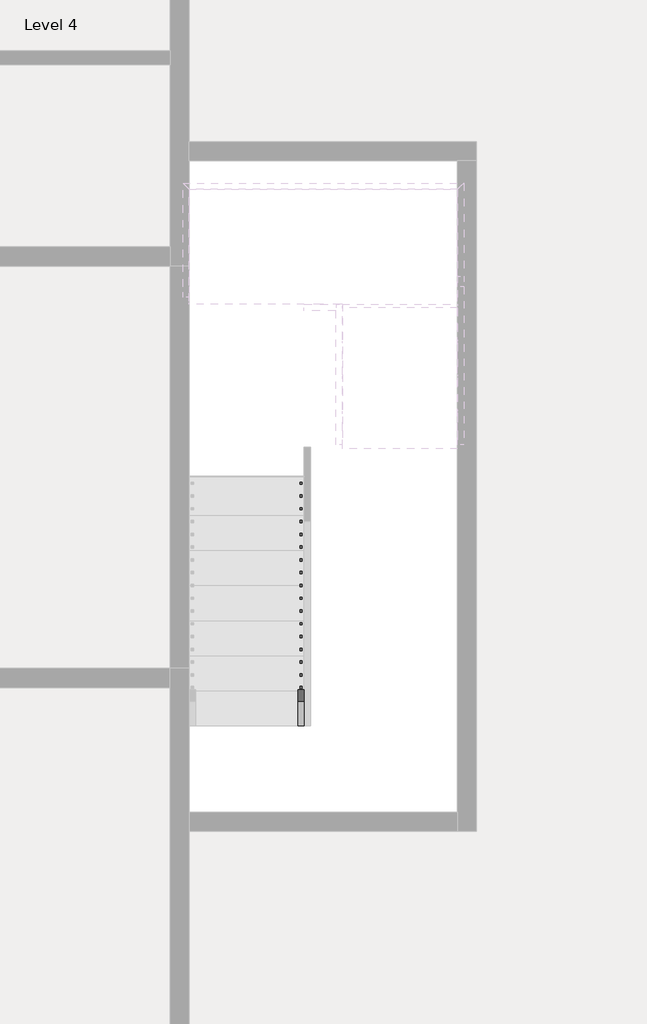
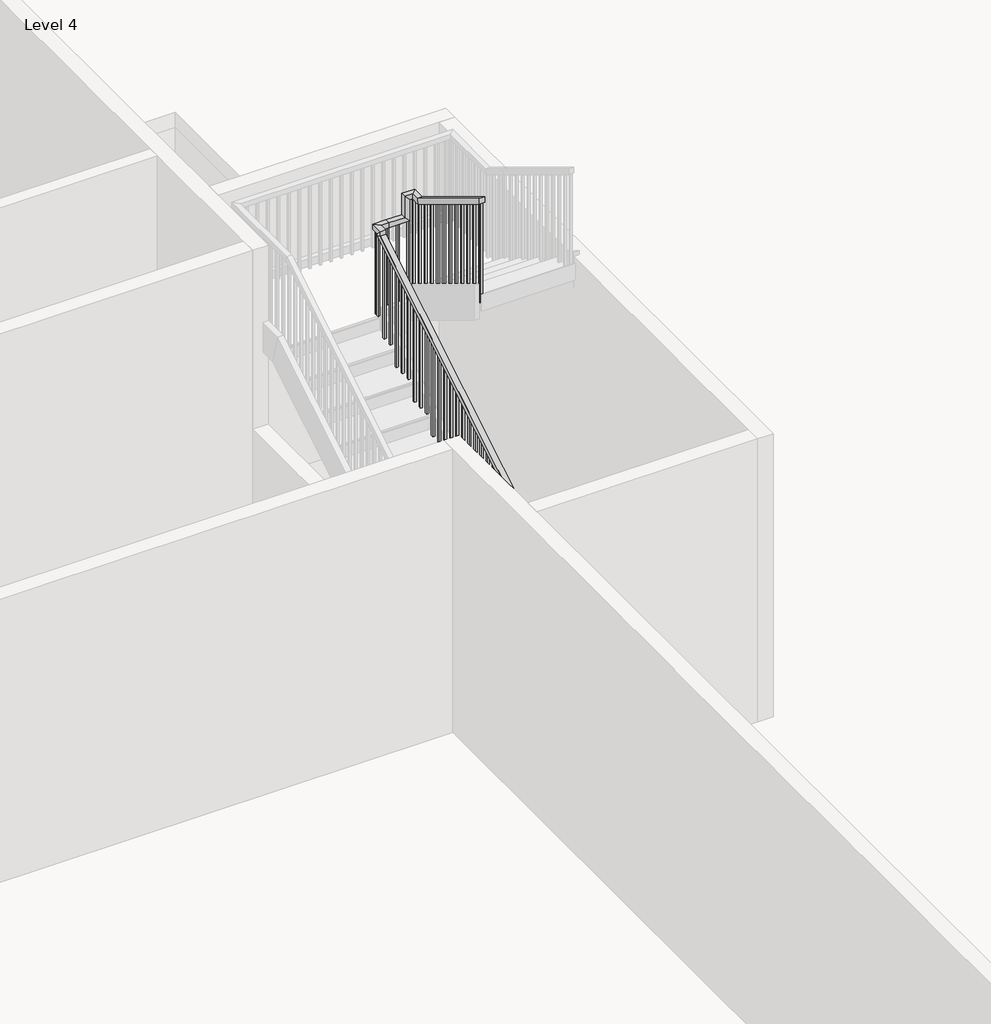
# One storey, part 7 of 8: 1 railing.
"""IFC4 building model written with IfcOpenShell, lengths in millimetres."""

from ifc_helpers import new_model, si_unit, frame, origin, place, context, project, spatial, polyline, outline, extrude, faceted_brep, element, save

model = new_model("IFC4")

# Units and contexts
model_context = context("Model", 3, world=origin())
ifc_project = project(units=[si_unit("LENGTHUNIT", "METRE", prefix="MILLI")], contexts=[model_context])

# Site, building, storey
site = spatial("IfcSite", under=ifc_project)
building = spatial("IfcBuilding", under=site)
storey = spatial("IfcBuildingStorey", under=building, Name="Level 4", Elevation=34378.6172466)

# Railing
placement = place(None, origin())
element("IfcRailing", 1, ObjectType="Handrail - Rectangular", at=placement, inside=storey, context=model_context, shape_type="SolidModel", body=[
    faceted_brep([(-2753.8415084, 19841.9216096, 35462.3505799), (-2753.8415084, 19841.9216096, 35402.9491197), (-2703.0415084, 19841.9216096, 35402.9491197), (-2703.0415084, 19841.9216096, 35462.3505799), (-2753.8415084, 23118.5216096, 37448.1687618), (-2753.8415084, 23169.3216096, 37419.5551803), (-2703.0415084, 23169.3216096, 37419.5551803), (-2703.0415084, 23118.5216096, 37448.1687618), (-2753.8415084, 23118.5216096, 37494.3505799), (-2753.8415084, 23169.3216096, 37443.5505799), (-2703.0415084, 23169.3216096, 37443.5505799), (-2703.0415084, 23118.5216096, 37494.3505799), (-2753.8415084, 23245.5216096, 37494.3505799), (-2753.8415084, 23245.5216096, 37443.5505799), (-2703.0415084, 23194.7216096, 37443.5505799), (-2703.0415084, 23194.7216096, 37494.3505799), (-2626.8415084, 23245.5216096, 37494.3505799), (-2626.8415084, 23245.5216096, 37443.5505799), (-2626.8415084, 23194.7216096, 37443.5505799), (-2626.8415084, 23194.7216096, 37494.3505799), (-2474.4415084, 23245.5216096, 37494.3505799), (-2423.6415084, 23245.5216096, 37443.5505799), (-2423.6415084, 23194.7216096, 37443.5505799), (-2474.4415084, 23194.7216096, 37494.3505799), (-2474.4415084, 23245.5216096, 37709.8657314), (-2423.6415084, 23245.5216096, 37659.0657314), (-2423.6415084, 23194.7216096, 37659.0657314), (-2474.4415084, 23194.7216096, 37709.8657314), (-2347.4415084, 23245.5216096, 37709.8657314), (-2347.4415084, 23245.5216096, 37659.0657314), (-2398.2415084, 23194.7216096, 37659.0657314), (-2398.2415084, 23194.7216096, 37709.8657314), (-2347.4415084, 23118.5216096, 37709.8657314), (-2347.4415084, 23104.3292002, 37659.0657314), (-2398.2415084, 23104.3292002, 37659.0657314), (-2398.2415084, 23118.5216096, 37709.8657314), (-2347.4415084, 22077.1216096, 38341.0172466), (-2398.2415084, 22077.1216096, 38341.0172466), (-2398.2415084, 22077.1216096, 38281.6157863), (-2347.4415084, 22077.1216096, 38281.6157863)], [[[0, 1, 2, 3]], [[1, 0, 4, 5]], [[2, 1, 5, 6]], [[3, 2, 6, 7]], [[0, 3, 7, 4]], [[5, 4, 8, 9]], [[6, 5, 9, 10]], [[7, 6, 10, 11]], [[4, 7, 11, 8]], [[9, 8, 12, 13]], [[10, 9, 13, 14]], [[11, 10, 14, 15]], [[8, 11, 15, 12]], [[13, 12, 16, 17]], [[14, 13, 17, 18]], [[15, 14, 18, 19]], [[12, 15, 19, 16]], [[17, 16, 20, 21]], [[18, 17, 21, 22]], [[19, 18, 22, 23]], [[16, 19, 23, 20]], [[21, 20, 24, 25]], [[22, 21, 25, 26]], [[23, 22, 26, 27]], [[20, 23, 27, 24]], [[25, 24, 28, 29]], [[26, 25, 29, 30]], [[27, 26, 30, 31]], [[24, 27, 31, 28]], [[29, 28, 32, 33]], [[30, 29, 33, 34]], [[31, 30, 34, 35]], [[28, 31, 35, 32]], [[36, 37, 38, 39]], [[33, 32, 36, 39]], [[34, 33, 39, 38]], [[35, 34, 38, 37]], [[32, 35, 37, 36]]]),
    extrude(outline(polyline([(22092.9966096, 38271.9945742), (22112.0466096, 38260.4491197), (22112.0466096, 37257.2839133), (22092.9966096, 37257.2839133), (22092.9966096, 38271.9945742)])), frame((-2382.3665084, 0.0, 0.0), z_axis=(1.0, 0.0, 0.0), x_axis=(0.0, 1.0, 0.0)), (0.0, 0.0, 1.0), 19.05),
    extrude(outline(polyline([(22194.5966096, 38210.4188166), (22213.6466096, 38198.8733621), (22213.6466096, 37257.2839133), (22194.5966096, 37257.2839133), (22194.5966096, 38210.4188166)])), frame((-2382.3665084, 0.0, 0.0), z_axis=(1.0, 0.0, 0.0), x_axis=(0.0, 1.0, 0.0)), (0.0, 0.0, 1.0), 19.05),
    extrude(outline(polyline([(22296.1966096, 38148.8430591), (22315.2466096, 38137.2976045), (22315.2466096, 37257.2839133), (22296.1966096, 37257.2839133), (22296.1966096, 38148.8430591)])), frame((-2382.3665084, 0.0, 0.0), z_axis=(1.0, 0.0, 0.0), x_axis=(0.0, 1.0, 0.0)), (0.0, 0.0, 1.0), 19.05),
    extrude(outline(polyline([(22397.7966096, 38087.2673015), (22416.8466096, 38075.721847), (22416.8466096, 37087.9505799), (22397.7966096, 37087.9505799), (22397.7966096, 38087.2673015)])), frame((-2382.3665084, 0.0, 0.0), z_axis=(1.0, 0.0, 0.0), x_axis=(0.0, 1.0, 0.0)), (0.0, 0.0, 1.0), 19.05),
    extrude(outline(polyline([(22499.3966096, 38025.6915439), (22518.4466096, 38014.1460894), (22518.4466096, 37087.9505799), (22499.3966096, 37087.9505799), (22499.3966096, 38025.6915439)])), frame((-2382.3665084, 0.0, 0.0), z_axis=(1.0, 0.0, 0.0), x_axis=(0.0, 1.0, 0.0)), (0.0, 0.0, 1.0), 19.05),
    extrude(outline(polyline([(22600.9966096, 37964.1157863), (22620.0466096, 37952.5703318), (22620.0466096, 37087.9505799), (22600.9966096, 37087.9505799), (22600.9966096, 37964.1157863)])), frame((-2382.3665084, 0.0, 0.0), z_axis=(1.0, 0.0, 0.0), x_axis=(0.0, 1.0, 0.0)), (0.0, 0.0, 1.0), 19.05),
    extrude(outline(polyline([(22702.5966096, 37902.5400288), (22721.6466096, 37890.9945742), (22721.6466096, 36918.6172466), (22702.5966096, 36918.6172466), (22702.5966096, 37902.5400288)])), frame((-2382.3665084, 0.0, 0.0), z_axis=(1.0, 0.0, 0.0), x_axis=(0.0, 1.0, 0.0)), (0.0, 0.0, 1.0), 19.05),
    extrude(outline(polyline([(22804.1966096, 37840.9642712), (22823.2466096, 37829.4188166), (22823.2466096, 36918.6172466), (22804.1966096, 36918.6172466), (22804.1966096, 37840.9642712)])), frame((-2382.3665084, 0.0, 0.0), z_axis=(1.0, 0.0, 0.0), x_axis=(0.0, 1.0, 0.0)), (0.0, 0.0, 1.0), 19.05),
    extrude(outline(polyline([(22905.7966096, 37779.3885136), (22924.8466096, 37767.8430591), (22924.8466096, 36918.6172466), (22905.7966096, 36918.6172466), (22905.7966096, 37779.3885136)])), frame((-2382.3665084, 0.0, 0.0), z_axis=(1.0, 0.0, 0.0), x_axis=(0.0, 1.0, 0.0)), (0.0, 0.0, 1.0), 19.05),
    extrude(outline(polyline([(23007.3966096, 37717.812756), (23026.4466096, 37706.2673015), (23026.4466096, 36749.2839133), (23007.3966096, 36749.2839133), (23007.3966096, 37717.812756)])), frame((-2382.3665084, 0.0, 0.0), z_axis=(1.0, 0.0, 0.0), x_axis=(0.0, 1.0, 0.0)), (0.0, 0.0, 1.0), 19.05),
    extrude(outline(polyline([(23108.9966096, 37656.2369985), (23128.0466096, 37644.6915439), (23128.0466096, 36749.2839133), (23108.9966096, 36749.2839133), (23108.9966096, 37656.2369985)])), frame((-2382.3665084, 0.0, 0.0), z_axis=(1.0, 0.0, 0.0), x_axis=(0.0, 1.0, 0.0)), (0.0, 0.0, 1.0), 19.05),
    extrude(outline(polyline([(-2433.1665084, 23210.5966096), (-2433.1665084, 23229.6466096), (-2414.1165084, 23229.6466096), (-2414.1165084, 23210.5966096), (-2433.1665084, 23210.5966096)])), frame((0.0, 0.0, 36579.9505799), z_axis=(0.0, 0.0, 1.0), x_axis=(1.0, 0.0, 0.0)), (0.0, 0.0, 1.0), 1079.1151515),
    extrude(outline(polyline([(-2534.7665084, 23210.5966096), (-2534.7665084, 23229.6466096), (-2515.7165084, 23229.6466096), (-2515.7165084, 23210.5966096), (-2534.7665084, 23210.5966096)])), frame((0.0, 0.0, 36579.9505799), z_axis=(0.0, 0.0, 1.0), x_axis=(1.0, 0.0, 0.0)), (0.0, 0.0, 1.0), 863.6),
    extrude(outline(polyline([(-2636.3665084, 23210.5966096), (-2636.3665084, 23229.6466096), (-2617.3165084, 23229.6466096), (-2617.3165084, 23210.5966096), (-2636.3665084, 23210.5966096)])), frame((0.0, 0.0, 36579.9505799), z_axis=(0.0, 0.0, 1.0), x_axis=(1.0, 0.0, 0.0)), (0.0, 0.0, 1.0), 863.6),
    extrude(outline(polyline([(-2718.9165084, 23185.1966096), (-2737.9665084, 23185.1966096), (-2737.9665084, 23204.2466096), (-2718.9165084, 23204.2466096), (-2718.9165084, 23185.1966096)])), frame((0.0, 0.0, 36579.9505799), z_axis=(0.0, 0.0, 1.0), x_axis=(1.0, 0.0, 0.0)), (0.0, 0.0, 1.0), 863.6),
    extrude(outline(polyline([(23083.5966096, 37367.6006348), (23102.6466096, 37379.1460894), (23102.6466096, 36410.6172466), (23083.5966096, 36410.6172466), (23083.5966096, 37367.6006348)])), frame((-2737.9665084, 0.0, 0.0), z_axis=(1.0, 0.0, 0.0), x_axis=(0.0, 1.0, 0.0)), (0.0, 0.0, 1.0), 19.05),
    extrude(outline(polyline([(22981.9966096, 37306.0248773), (23001.0466096, 37317.5703318), (23001.0466096, 36410.6172466), (22981.9966096, 36410.6172466), (22981.9966096, 37306.0248773)])), frame((-2737.9665084, 0.0, 0.0), z_axis=(1.0, 0.0, 0.0), x_axis=(0.0, 1.0, 0.0)), (0.0, 0.0, 1.0), 19.05),
    extrude(outline(polyline([(22880.3966096, 37244.4491197), (22899.4466096, 37255.9945742), (22899.4466096, 36241.2839133), (22880.3966096, 36241.2839133), (22880.3966096, 37244.4491197)])), frame((-2737.9665084, 0.0, 0.0), z_axis=(1.0, 0.0, 0.0), x_axis=(0.0, 1.0, 0.0)), (0.0, 0.0, 1.0), 19.05),
    extrude(outline(polyline([(22778.7966096, 37182.8733621), (22797.8466096, 37194.4188166), (22797.8466096, 36241.2839133), (22778.7966096, 36241.2839133), (22778.7966096, 37182.8733621)])), frame((-2737.9665084, 0.0, 0.0), z_axis=(1.0, 0.0, 0.0), x_axis=(0.0, 1.0, 0.0)), (0.0, 0.0, 1.0), 19.05),
    extrude(outline(polyline([(22677.1966096, 37121.2976045), (22696.2466096, 37132.8430591), (22696.2466096, 36241.2839133), (22677.1966096, 36241.2839133), (22677.1966096, 37121.2976045)])), frame((-2737.9665084, 0.0, 0.0), z_axis=(1.0, 0.0, 0.0), x_axis=(0.0, 1.0, 0.0)), (0.0, 0.0, 1.0), 19.05),
    extrude(outline(polyline([(22575.5966096, 37059.721847), (22594.6466096, 37071.2673015), (22594.6466096, 36071.9505799), (22575.5966096, 36071.9505799), (22575.5966096, 37059.721847)])), frame((-2737.9665084, 0.0, 0.0), z_axis=(1.0, 0.0, 0.0), x_axis=(0.0, 1.0, 0.0)), (0.0, 0.0, 1.0), 19.05),
    extrude(outline(polyline([(22473.9966096, 36998.1460894), (22493.0466096, 37009.6915439), (22493.0466096, 36071.9505799), (22473.9966096, 36071.9505799), (22473.9966096, 36998.1460894)])), frame((-2737.9665084, 0.0, 0.0), z_axis=(1.0, 0.0, 0.0), x_axis=(0.0, 1.0, 0.0)), (0.0, 0.0, 1.0), 19.05),
    extrude(outline(polyline([(22372.3966096, 36936.5703318), (22391.4466096, 36948.1157863), (22391.4466096, 36071.9505799), (22372.3966096, 36071.9505799), (22372.3966096, 36936.5703318)])), frame((-2737.9665084, 0.0, 0.0), z_axis=(1.0, 0.0, 0.0), x_axis=(0.0, 1.0, 0.0)), (0.0, 0.0, 1.0), 19.05),
    extrude(outline(polyline([(22270.7966096, 36874.9945742), (22289.8466096, 36886.5400288), (22289.8466096, 35902.6172466), (22270.7966096, 35902.6172466), (22270.7966096, 36874.9945742)])), frame((-2737.9665084, 0.0, 0.0), z_axis=(1.0, 0.0, 0.0), x_axis=(0.0, 1.0, 0.0)), (0.0, 0.0, 1.0), 19.05),
    extrude(outline(polyline([(22169.1966096, 36813.4188166), (22188.2466096, 36824.9642712), (22188.2466096, 35902.6172466), (22169.1966096, 35902.6172466), (22169.1966096, 36813.4188166)])), frame((-2737.9665084, 0.0, 0.0), z_axis=(1.0, 0.0, 0.0), x_axis=(0.0, 1.0, 0.0)), (0.0, 0.0, 1.0), 19.05),
    extrude(outline(polyline([(22067.5966096, 36751.8430591), (22086.6466096, 36763.3885136), (22086.6466096, 35902.6172466), (22067.5966096, 35902.6172466), (22067.5966096, 36751.8430591)])), frame((-2737.9665084, 0.0, 0.0), z_axis=(1.0, 0.0, 0.0), x_axis=(0.0, 1.0, 0.0)), (0.0, 0.0, 1.0), 19.05),
    extrude(outline(polyline([(21965.9966096, 36690.2673015), (21985.0466096, 36701.812756), (21985.0466096, 35733.2839133), (21965.9966096, 35733.2839133), (21965.9966096, 36690.2673015)])), frame((-2737.9665084, 0.0, 0.0), z_axis=(1.0, 0.0, 0.0), x_axis=(0.0, 1.0, 0.0)), (0.0, 0.0, 1.0), 19.05),
    extrude(outline(polyline([(21864.3966096, 36628.6915439), (21883.4466096, 36640.2369985), (21883.4466096, 35733.2839133), (21864.3966096, 35733.2839133), (21864.3966096, 36628.6915439)])), frame((-2737.9665084, 0.0, 0.0), z_axis=(1.0, 0.0, 0.0), x_axis=(0.0, 1.0, 0.0)), (0.0, 0.0, 1.0), 19.05),
    extrude(outline(polyline([(21762.7966096, 36567.1157863), (21781.8466096, 36578.6612409), (21781.8466096, 35563.9505799), (21762.7966096, 35563.9505799), (21762.7966096, 36567.1157863)])), frame((-2737.9665084, 0.0, 0.0), z_axis=(1.0, 0.0, 0.0), x_axis=(0.0, 1.0, 0.0)), (0.0, 0.0, 1.0), 19.05),
    extrude(outline(polyline([(21661.1966096, 36505.5400288), (21680.2466096, 36517.0854833), (21680.2466096, 35563.9505799), (21661.1966096, 35563.9505799), (21661.1966096, 36505.5400288)])), frame((-2737.9665084, 0.0, 0.0), z_axis=(1.0, 0.0, 0.0), x_axis=(0.0, 1.0, 0.0)), (0.0, 0.0, 1.0), 19.05),
    extrude(outline(polyline([(21559.5966096, 36443.9642712), (21578.6466096, 36455.5097257), (21578.6466096, 35563.9505799), (21559.5966096, 35563.9505799), (21559.5966096, 36443.9642712)])), frame((-2737.9665084, 0.0, 0.0), z_axis=(1.0, 0.0, 0.0), x_axis=(0.0, 1.0, 0.0)), (0.0, 0.0, 1.0), 19.05),
    extrude(outline(polyline([(21457.9966096, 36382.3885136), (21477.0466096, 36393.9339682), (21477.0466096, 35394.6172466), (21457.9966096, 35394.6172466), (21457.9966096, 36382.3885136)])), frame((-2737.9665084, 0.0, 0.0), z_axis=(1.0, 0.0, 0.0), x_axis=(0.0, 1.0, 0.0)), (0.0, 0.0, 1.0), 19.05),
    extrude(outline(polyline([(21356.3966096, 36320.812756), (21375.4466096, 36332.3582106), (21375.4466096, 35394.6172466), (21356.3966096, 35394.6172466), (21356.3966096, 36320.812756)])), frame((-2737.9665084, 0.0, 0.0), z_axis=(1.0, 0.0, 0.0), x_axis=(0.0, 1.0, 0.0)), (0.0, 0.0, 1.0), 19.05),
    extrude(outline(polyline([(21254.7966096, 36259.2369985), (21273.8466096, 36270.782453), (21273.8466096, 35394.6172466), (21254.7966096, 35394.6172466), (21254.7966096, 36259.2369985)])), frame((-2737.9665084, 0.0, 0.0), z_axis=(1.0, 0.0, 0.0), x_axis=(0.0, 1.0, 0.0)), (0.0, 0.0, 1.0), 19.05),
    extrude(outline(polyline([(21153.1966096, 36197.6612409), (21172.2466096, 36209.2066954), (21172.2466096, 35225.2839133), (21153.1966096, 35225.2839133), (21153.1966096, 36197.6612409)])), frame((-2737.9665084, 0.0, 0.0), z_axis=(1.0, 0.0, 0.0), x_axis=(0.0, 1.0, 0.0)), (0.0, 0.0, 1.0), 19.05),
    extrude(outline(polyline([(21051.5966096, 36136.0854833), (21070.6466096, 36147.6309379), (21070.6466096, 35225.2839133), (21051.5966096, 35225.2839133), (21051.5966096, 36136.0854833)])), frame((-2737.9665084, 0.0, 0.0), z_axis=(1.0, 0.0, 0.0), x_axis=(0.0, 1.0, 0.0)), (0.0, 0.0, 1.0), 19.05),
    extrude(outline(polyline([(20949.9966096, 36074.5097257), (20969.0466096, 36086.0551803), (20969.0466096, 35225.2839133), (20949.9966096, 35225.2839133), (20949.9966096, 36074.5097257)])), frame((-2737.9665084, 0.0, 0.0), z_axis=(1.0, 0.0, 0.0), x_axis=(0.0, 1.0, 0.0)), (0.0, 0.0, 1.0), 19.05),
    extrude(outline(polyline([(20848.3966096, 36012.9339682), (20867.4466096, 36024.4794227), (20867.4466096, 35055.9505799), (20848.3966096, 35055.9505799), (20848.3966096, 36012.9339682)])), frame((-2737.9665084, 0.0, 0.0), z_axis=(1.0, 0.0, 0.0), x_axis=(0.0, 1.0, 0.0)), (0.0, 0.0, 1.0), 19.05),
    extrude(outline(polyline([(20746.7966096, 35951.3582106), (20765.8466096, 35962.9036651), (20765.8466096, 35055.9505799), (20746.7966096, 35055.9505799), (20746.7966096, 35951.3582106)])), frame((-2737.9665084, 0.0, 0.0), z_axis=(1.0, 0.0, 0.0), x_axis=(0.0, 1.0, 0.0)), (0.0, 0.0, 1.0), 19.05),
    extrude(outline(polyline([(20645.1966096, 35889.782453), (20664.2466096, 35901.3279076), (20664.2466096, 34886.6172466), (20645.1966096, 34886.6172466), (20645.1966096, 35889.782453)])), frame((-2737.9665084, 0.0, 0.0), z_axis=(1.0, 0.0, 0.0), x_axis=(0.0, 1.0, 0.0)), (0.0, 0.0, 1.0), 19.05),
    extrude(outline(polyline([(20543.5966096, 35828.2066954), (20562.6466096, 35839.75215), (20562.6466096, 34886.6172466), (20543.5966096, 34886.6172466), (20543.5966096, 35828.2066954)])), frame((-2737.9665084, 0.0, 0.0), z_axis=(1.0, 0.0, 0.0), x_axis=(0.0, 1.0, 0.0)), (0.0, 0.0, 1.0), 19.05),
    extrude(outline(polyline([(20441.9966096, 35766.6309379), (20461.0466096, 35778.1763924), (20461.0466096, 34886.6172466), (20441.9966096, 34886.6172466), (20441.9966096, 35766.6309379)])), frame((-2737.9665084, 0.0, 0.0), z_axis=(1.0, 0.0, 0.0), x_axis=(0.0, 1.0, 0.0)), (0.0, 0.0, 1.0), 19.05),
    extrude(outline(polyline([(20340.3966096, 35705.0551803), (20359.4466096, 35716.6006348), (20359.4466096, 34717.2839133), (20340.3966096, 34717.2839133), (20340.3966096, 35705.0551803)])), frame((-2737.9665084, 0.0, 0.0), z_axis=(1.0, 0.0, 0.0), x_axis=(0.0, 1.0, 0.0)), (0.0, 0.0, 1.0), 19.05),
    extrude(outline(polyline([(20238.7966096, 35643.4794227), (20257.8466096, 35655.0248773), (20257.8466096, 34717.2839133), (20238.7966096, 34717.2839133), (20238.7966096, 35643.4794227)])), frame((-2737.9665084, 0.0, 0.0), z_axis=(1.0, 0.0, 0.0), x_axis=(0.0, 1.0, 0.0)), (0.0, 0.0, 1.0), 19.05),
    extrude(outline(polyline([(20137.1966096, 35581.9036651), (20156.2466096, 35593.4491197), (20156.2466096, 34717.2839133), (20137.1966096, 34717.2839133), (20137.1966096, 35581.9036651)])), frame((-2737.9665084, 0.0, 0.0), z_axis=(1.0, 0.0, 0.0), x_axis=(0.0, 1.0, 0.0)), (0.0, 0.0, 1.0), 19.05),
    extrude(outline(polyline([(20035.5966096, 35520.3279076), (20054.6466096, 35531.8733621), (20054.6466096, 34547.9505799), (20035.5966096, 34547.9505799), (20035.5966096, 35520.3279076)])), frame((-2737.9665084, 0.0, 0.0), z_axis=(1.0, 0.0, 0.0), x_axis=(0.0, 1.0, 0.0)), (0.0, 0.0, 1.0), 19.05),
    extrude(outline(polyline([(19933.9966096, 35458.75215), (19953.0466096, 35470.2976045), (19953.0466096, 34547.9505799), (19933.9966096, 34547.9505799), (19933.9966096, 35458.75215)])), frame((-2737.9665084, 0.0, 0.0), z_axis=(1.0, 0.0, 0.0), x_axis=(0.0, 1.0, 0.0)), (0.0, 0.0, 1.0), 19.05),
    extrude(outline(polyline([(-2382.3665084, 23210.5966096), (-2382.3665084, 23229.6466096), (-2363.3165084, 23229.6466096), (-2363.3165084, 23210.5966096), (-2382.3665084, 23210.5966096)])), frame((0.0, 0.0, 36579.9505799), z_axis=(0.0, 0.0, 1.0), x_axis=(1.0, 0.0, 0.0)), (0.0, 0.0, 1.0), 1079.1151515),
    extrude(outline(polyline([(-2718.9165084, 23210.5966096), (-2737.9665084, 23210.5966096), (-2737.9665084, 23229.6466096), (-2718.9165084, 23229.6466096), (-2718.9165084, 23210.5966096)])), frame((0.0, 0.0, 36579.9505799), z_axis=(0.0, 0.0, 1.0), x_axis=(1.0, 0.0, 0.0)), (0.0, 0.0, 1.0), 863.6),
    extrude(outline(polyline([(22077.1216096, 38281.6157863), (22096.1716096, 38270.0703318), (22096.1716096, 37257.2839133), (22077.1216096, 37257.2839133), (22077.1216096, 38281.6157863)])), frame((-2382.3665084, 0.0, 0.0), z_axis=(1.0, 0.0, 0.0), x_axis=(0.0, 1.0, 0.0)), (0.0, 0.0, 1.0), 19.05),
    extrude(outline(polyline([(19841.9216096, 35402.9491197), (19860.9716096, 35414.4945742), (19860.9716096, 34547.9505799), (19841.9216096, 34547.9505799), (19841.9216096, 35402.9491197)])), frame((-2737.9665084, 0.0, 0.0), z_axis=(1.0, 0.0, 0.0), x_axis=(0.0, 1.0, 0.0)), (0.0, 0.0, 1.0), 19.05),
])

save(model, "model.ifc")

# Revit data of these elements
# Type "Handrail - Rectangular"
#   Assembly Code = "C2010400"
#   built-in parameter 1008612 = 0.0416667 (stored number, unit not read)
#   built-in parameter 1008611 = 0.0416667 (stored number, unit not read)
#   built-in parameter 1008609 = 0.333333 (stored number, unit not read)
#   built-in parameter 1008604 = 0.166667 (stored number, unit not read)
#   built-in parameter 1008603 = 0.166667 (stored number, unit not read)
#   Railing Height = 3' - 0"
#   built-in parameter 1008630 = 2
#   built-in parameter 1008610 = 2
#   built-in parameter 1008618 = Baluster - Square : 3/4"
# Element 1 (IfcRailing, "Handrail - Rectangular")
#   Phase Created = New Construction
